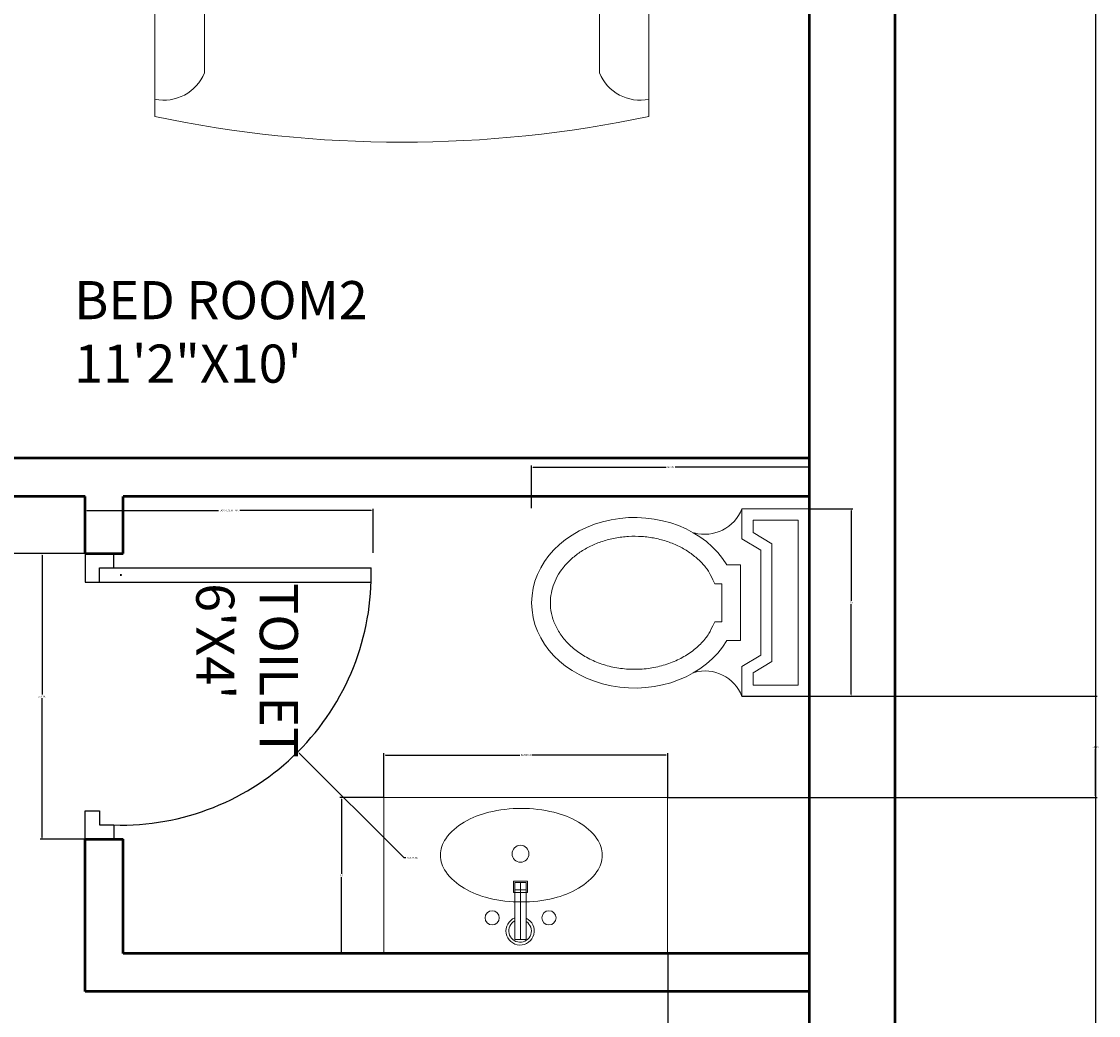
# Model space of a CAD drawing. Units: inches. Extents: x 1798 to 2141, y 1923 to 2386.
# Tile 8 of 9: x 2028 to 2141, y 2177 to 2281. Entities that reach past the tile are written whole.
import ezdxf

# ---------------------------------------------------------------- set-up
doc = ezdxf.new("R2010")
doc.units = ezdxf.units.IN
for name, color, linetype, lineweight in [('A-ANNO-DIMS', 2, 'Continuous', 18), ('A-AREA-IDEN', 7, 'Continuous', 25), ('A-FLOR-FIXT', 9, 'Continuous', 18), ('A-FURN', 8, 'Continuous', 13), ('door', 40, 'Continuous', 25), ('wall', 4, 'Continuous', 50)]:
    doc.layers.add(name, color=color, linetype=linetype, lineweight=lineweight)
doc.styles.get("Standard").update_dxf_attribs({"font": 'arial.ttf'})
doc.dimstyles.get("Standard").update_dxf_attribs({"dimtxt": 0.18, "dimasz": 0.18, "dimexe": 0.18, "dimexo": 0.0625, "dimgap": 0.09, "dimtad": 0, "dimtih": 1, "dimtoh": 1, "dimdec": 4, "dimzin": 0, "dimdsep": 46, "dimtxsty": 'Standard', "dimcen": 0.09, "dimadec": 0, "dimazin": 0, "dimtfac": 1, "dimtdec": 4, "dimtofl": 0, "dimtmove": 0, "dimatfit": 3, "dimfxl": 1, "dimtolj": 1, "dimtzin": 0, "dimarcsym": 0})

# ---------------------------------------------------------------- blocks, each defined once
blk = doc.blocks.new('A$C4F543DC7')
for p, q in [((0.2381, 3.1233, -0.4388), (0.2381, 3.3614, -0.4388)), ((3.0888, 3.1233, -0.4388), (3.0888, 3.3614, -0.4388)), ((0.0134, 3.35, -0.1688), (3.3134, 3.35, -0.1688)), ((0.4634, 3.35, -0.1688), (0.0134, 3.35, -0.1688)), ((0.0134, 2.896, -0.1688), (0.0134, 3.35, -0.1688)), ((0.0134, 3.35, -0.1688), (0.0134, 2.896, -0.1688)), ((0.4634, 3.35, -0.1688), (0.4634, 0.8, -0.1688)), ((2.8634, 3.35, -0.1688), (0.4634, 3.35, -0.1688)), ((0.4634, 2.896, -0.1688), (0.4634, 3.35, -0.1688)), ((2.8634, 0.8, -0.1688), (2.8634, 3.35, -0.1688)), ((2.8634, 3.35, -0.1688), (3.3134, 3.35, -0.1688)), ((2.8634, 2.896, -0.1688), (2.8634, 3.35, -0.1688)), ((3.3134, 3.35, -0.1688), (3.3134, 2.896, -0.1688)), ((3.3134, 3.35, -0.1688), (3.3134, 2.896, -0.1688)), ((1.5354, 3.226, -0.1688), (0.6684, 3.226, -0.1688)), ((2.6644, 3.226, -0.1688), (1.7974, 3.226, -0.1688)), ((0.2381, 3.1233, -0.4388), (0, 3.1233, -0.4388)), ((0.2381, 3.1233, -0.4388), (0.4762, 3.1233, -0.4388)), ((0.2381, 3.1233, -0.4388), (0.2381, 2.8852, -0.4388)), ((0.5684, 3.126, -0.1688), (0.5684, 2.884, -0.1688)), ((1.6354, 2.884, -0.1688), (1.6354, 3.126, -0.1688)), ((1.6974, 3.126, -0.1688), (1.6974, 2.884, -0.1688)), ((2.7644, 2.884, -0.1688), (2.7644, 3.126, -0.1688)), ((3.0888, 3.1233, -0.4388), (2.8507, 3.1233, -0.4388)), ((3.0888, 3.1233, -0.4388), (3.0888, 2.8852, -0.4388)), ((3.0888, 3.1233, -0.4388), (3.3269, 3.1233, -0.4388)), ((0.4634, 2.896, -0.1688), (0.0134, 2.896, -0.1688)), ((0.0134, 2.896, -0.1688), (0.4634, 2.896, -0.1688)), ((0.4634, 0.8, -0.1688), (0.4634, 2.896, -0.1688)), ((2.8634, 2.896, -0.1688), (2.8634, 0.8, -0.1688)), ((3.3134, 2.896, -0.1688), (2.8634, 2.896, -0.1688)), ((3.3134, 2.896, -0.1688), (2.8634, 2.896, -0.1688)), ((0.6684, 2.784, -0.1688), (1.5354, 2.784, -0.1688)), ((1.7974, 2.784, -0.1688), (2.6644, 2.784, -0.1688)), ((1.6534, 2.573, -0.1688), (0.5504, 2.025, -0.1688)), ((0.8414, 1.752, -0.1688), (1.6534, 2.573, -0.1688)), ((2.4814, 1.752, -0.1688), (1.6694, 2.573, -0.1688)), ((1.6694, 2.573, -0.1688), (2.7724, 2.025, -0.1688)), ((0.5504, 2.025, -0.1688), (0.8414, 1.752, -0.1688)), ((2.7724, 2.025, -0.1688), (2.4814, 1.752, -0.1688)), ((2.683, 1.312, -0.1688), (2.7182, 1.3641, -0.1688)), ((0.5369, 1.3267, -0.1688), (0.6088, 1.2835, -0.1688)), ((2.6479, 1.2774, -0.1688), (2.683, 1.312, -0.1688)), ((0.6088, 1.2835, -0.1688), (0.6756, 1.2566, -0.1688)), ((1.3963, 1.2612, -0.1688), (1.4328, 1.2664, -0.1688)), ((1.4328, 1.2664, -0.1688), (1.4679, 1.2677, -0.1688)), ((1.4679, 1.2677, -0.1688), (1.501, 1.2643, -0.1688)), ((1.8849, 1.263, -0.1688), (1.913, 1.2698, -0.1688)), ((1.913, 1.2698, -0.1688), (1.9397, 1.2722, -0.1688)), ((1.9397, 1.2722, -0.1688), (1.9649, 1.2692, -0.1688)), ((1.9649, 1.2692, -0.1688), (1.989, 1.2617, -0.1688)), ((2.6129, 1.257, -0.1688), (2.6479, 1.2774, -0.1688)), ((0.6756, 1.2566, -0.1688), (0.7373, 1.2428, -0.1688)), ((0.7373, 1.2428, -0.1688), (0.794, 1.239, -0.1688)), ((0.794, 1.239, -0.1688), (0.8457, 1.242, -0.1688)), ((0.8457, 1.242, -0.1688), (0.8925, 1.2489, -0.1688)), ((0.8925, 1.2489, -0.1688), (0.9345, 1.2564, -0.1688)), ((0.9345, 1.2564, -0.1688), (0.9718, 1.2615, -0.1688)), ((0.9718, 1.2615, -0.1688), (1.0044, 1.2617, -0.1688)), ((1.0044, 1.2617, -0.1688), (1.0334, 1.2578, -0.1688)), ((1.0334, 1.2578, -0.1688), (1.0597, 1.2509, -0.1688)), ((1.0597, 1.2509, -0.1688), (1.0842, 1.2424, -0.1688)), ((1.0842, 1.2424, -0.1688), (1.1081, 1.2336, -0.1688)), ((1.1081, 1.2336, -0.1688), (1.1322, 1.2257, -0.1688)), ((1.1322, 1.2257, -0.1688), (1.1577, 1.2201, -0.1688)), ((1.2163, 1.2204, -0.1688), (1.2498, 1.2264, -0.1688)), ((1.2498, 1.2264, -0.1688), (1.2852, 1.2347, -0.1688)), ((1.2852, 1.2347, -0.1688), (1.3218, 1.2441, -0.1688)), ((1.3218, 1.2441, -0.1688), (1.3591, 1.2533, -0.1688)), ((1.3591, 1.2533, -0.1688), (1.3963, 1.2612, -0.1688)), ((1.501, 1.2643, -0.1688), (1.5324, 1.257, -0.1688)), ((1.5324, 1.257, -0.1688), (1.5624, 1.2473, -0.1688)), ((1.5624, 1.2473, -0.1688), (1.5915, 1.2365, -0.1688)), ((1.5915, 1.2365, -0.1688), (1.6199, 1.2259, -0.1688)), ((1.6199, 1.2259, -0.1688), (1.6481, 1.2169, -0.1688)), ((1.7651, 1.2199, -0.1688), (1.7955, 1.2301, -0.1688)), ((1.7955, 1.2301, -0.1688), (1.8258, 1.2417, -0.1688)), ((1.8258, 1.2417, -0.1688), (1.8557, 1.2531, -0.1688)), ((1.8557, 1.2531, -0.1688), (1.8849, 1.263, -0.1688)), ((1.989, 1.2617, -0.1688), (2.0124, 1.2512, -0.1688)), ((2.0124, 1.2512, -0.1688), (2.0359, 1.2391, -0.1688)), ((2.0359, 1.2391, -0.1688), (2.0599, 1.2269, -0.1688)), ((2.0599, 1.2269, -0.1688), (2.0849, 1.216, -0.1688)), ((2.242, 1.2182, -0.1688), (2.2791, 1.2279, -0.1688)), ((2.2791, 1.2279, -0.1688), (2.3173, 1.2378, -0.1688)), ((2.3173, 1.2378, -0.1688), (2.3558, 1.2465, -0.1688)), ((2.3558, 1.2465, -0.1688), (2.3944, 1.2527, -0.1688)), ((2.3944, 1.2527, -0.1688), (2.4325, 1.255, -0.1688)), ((2.4325, 1.255, -0.1688), (2.4698, 1.2529, -0.1688)), ((2.4698, 1.2529, -0.1688), (2.5064, 1.2488, -0.1688)), ((2.5064, 1.2488, -0.1688), (2.5423, 1.2459, -0.1688)), ((2.5423, 1.2459, -0.1688), (2.5777, 1.2476, -0.1688)), ((2.5777, 1.2476, -0.1688), (2.6129, 1.257, -0.1688)), ((0.6743, 1.1706, -0.1688), (0.7364, 1.1825, -0.1688)), ((0.7364, 1.1825, -0.1688), (0.7931, 1.1846, -0.1688)), ((0.7931, 1.1846, -0.1688), (0.8447, 1.1799, -0.1688)), ((0.8447, 1.1799, -0.1688), (0.8913, 1.1716, -0.1688)), ((1.0831, 1.172, -0.1688), (1.1072, 1.18, -0.1688)), ((1.1072, 1.18, -0.1688), (1.1316, 1.1872, -0.1688)), ((1.1316, 1.1872, -0.1688), (1.1573, 1.192, -0.1688)), ((1.1573, 1.192, -0.1688), (1.1851, 1.1932, -0.1688)), ((1.1577, 1.2201, -0.1688), (1.1855, 1.218, -0.1688)), ((1.1851, 1.1932, -0.1688), (1.2158, 1.1898, -0.1688)), ((1.1855, 1.218, -0.1688), (1.2163, 1.2204, -0.1688)), ((1.2158, 1.1898, -0.1688), (1.2491, 1.1828, -0.1688)), ((1.2491, 1.1828, -0.1688), (1.2842, 1.1734, -0.1688)), ((1.6191, 1.1716, -0.1688), (1.6475, 1.1797, -0.1688)), ((1.6475, 1.1797, -0.1688), (1.676, 1.1849, -0.1688)), ((1.6481, 1.2169, -0.1688), (1.6765, 1.2108, -0.1688)), ((1.676, 1.1849, -0.1688), (1.7049, 1.1858, -0.1688)), ((1.6765, 1.2108, -0.1688), (1.7053, 1.209, -0.1688)), ((1.7049, 1.1858, -0.1688), (1.7344, 1.1816, -0.1688)), ((1.7053, 1.209, -0.1688), (1.7349, 1.2124, -0.1688)), ((1.7344, 1.1816, -0.1688), (1.7643, 1.1731, -0.1688)), ((1.7349, 1.2124, -0.1688), (1.7651, 1.2199, -0.1688)), ((2.0849, 1.216, -0.1688), (2.1117, 1.2077, -0.1688)), ((2.1112, 1.1743, -0.1688), (2.1403, 1.1775, -0.1688)), ((2.1117, 1.2077, -0.1688), (2.1407, 1.2037, -0.1688)), ((2.1403, 1.1775, -0.1688), (2.1718, 1.1755, -0.1688)), ((2.1407, 1.2037, -0.1688), (2.1723, 1.2047, -0.1688)), ((2.1723, 1.2047, -0.1688), (2.2062, 1.21, -0.1688)), ((2.2062, 1.21, -0.1688), (2.242, 1.2182, -0.1688)), ((0.5334, 1.105, -0.1688), (0.6067, 1.1458, -0.1688)), ((0.6067, 1.1458, -0.1688), (0.6743, 1.1706, -0.1688)), ((0.8913, 1.1716, -0.1688), (0.9331, 1.1628, -0.1688)), ((0.9331, 1.1628, -0.1688), (0.9701, 1.1565, -0.1688)), ((0.9701, 1.1565, -0.1688), (1.0027, 1.1552, -0.1688)), ((1.0027, 1.1552, -0.1688), (1.0318, 1.1582, -0.1688)), ((1.0318, 1.1582, -0.1688), (1.0583, 1.1642, -0.1688)), ((1.0583, 1.1642, -0.1688), (1.0831, 1.172, -0.1688)), ((1.2842, 1.1734, -0.1688), (1.3206, 1.1629, -0.1688)), ((1.3206, 1.1629, -0.1688), (1.3575, 1.1524, -0.1688)), ((1.3575, 1.1524, -0.1688), (1.3945, 1.1434, -0.1688)), ((1.3945, 1.1434, -0.1688), (1.4308, 1.1371, -0.1688)), ((1.4308, 1.1371, -0.1688), (1.4658, 1.1347, -0.1688)), ((1.4658, 1.1347, -0.1688), (1.499, 1.137, -0.1688)), ((1.499, 1.137, -0.1688), (1.5306, 1.1433, -0.1688)), ((1.5306, 1.1433, -0.1688), (1.5609, 1.152, -0.1688)), ((1.5609, 1.152, -0.1688), (1.5903, 1.1619, -0.1688)), ((1.5903, 1.1619, -0.1688), (1.6191, 1.1716, -0.1688)), ((1.7643, 1.1731, -0.1688), (1.7944, 1.1619, -0.1688)), ((1.7944, 1.1619, -0.1688), (1.8244, 1.1494, -0.1688)), ((1.8244, 1.1494, -0.1688), (1.8539, 1.137, -0.1688)), ((1.8539, 1.137, -0.1688), (1.8827, 1.1263, -0.1688)), ((1.9868, 1.1243, -0.1688), (2.0106, 1.134, -0.1688)), ((2.0106, 1.134, -0.1688), (2.0344, 1.1454, -0.1688)), ((2.0344, 1.1454, -0.1688), (2.0588, 1.1568, -0.1688)), ((2.0588, 1.1568, -0.1688), (2.0842, 1.167, -0.1688)), ((2.0842, 1.167, -0.1688), (2.1112, 1.1743, -0.1688)), ((2.1718, 1.1755, -0.1688), (2.2056, 1.1691, -0.1688)), ((2.2056, 1.1691, -0.1688), (2.2411, 1.1598, -0.1688)), ((2.2411, 1.1598, -0.1688), (2.2779, 1.1489, -0.1688)), ((2.2779, 1.1489, -0.1688), (2.3157, 1.1379, -0.1688)), ((2.3157, 1.1379, -0.1688), (2.354, 1.1279, -0.1688)), ((1.8827, 1.1263, -0.1688), (1.9106, 1.1186, -0.1688)), ((1.9106, 1.1186, -0.1688), (1.9373, 1.1153, -0.1688)), ((1.9373, 1.1153, -0.1688), (1.9625, 1.1176, -0.1688)), ((1.9625, 1.1176, -0.1688), (1.9868, 1.1243, -0.1688)), ((2.354, 1.1279, -0.1688), (2.3923, 1.1205, -0.1688)), ((2.3923, 1.1205, -0.1688), (2.4304, 1.117, -0.1688)), ((2.4304, 1.117, -0.1688), (2.4677, 1.118, -0.1688)), ((2.4677, 1.118, -0.1688), (2.5043, 1.1209, -0.1688)), ((2.5043, 1.1209, -0.1688), (2.5403, 1.1226, -0.1688)), ((2.5403, 1.1226, -0.1688), (2.5757, 1.1199, -0.1688)), ((2.5757, 1.1199, -0.1688), (2.6106, 1.1094, -0.1688)), ((2.6106, 1.1094, -0.1688), (2.645, 1.0879, -0.1688)), ((2.645, 1.0879, -0.1688), (2.6789, 1.0522, -0.1688)), ((2.6789, 1.0522, -0.1688), (2.7124, 0.999, -0.1688)), ((0.4634, 0.85, -0.1688), (2.8634, 0.85, -0.1688)), ((0.4634, 0.8, -0.1688), (2.8634, 0.8, -0.1688)), ((0.6634, 0.8, -0.1688), (0.4634, 0.8, -0.1688)), ((0.6634, 0.8, -0.1688), (2.6634, 0.8, -0.1688)), ((0.6634, 0.104, -0.1688), (0.6634, 0.8, -0.1688)), ((0.6634, 0.104, -0.1688), (0.6634, 0.8, -0.1688)), ((0.8634, 0.281, -0.1688), (0.8634, 0.8, -0.1688)), ((2.4634, 0.8, -0.1688), (2.4634, 0.281, -0.1688)), ((2.8634, 0.8, -0.1688), (2.6634, 0.8, -0.1688)), ((2.6634, 0.8, -0.1688), (2.6634, 0.104, -0.1688)), ((2.6634, 0.8, -0.1688), (2.6634, 0.104, -0.1688))]:
    blk.add_line(p, q)
for centre, radius in [((0.2381, 3.1233, -0.4388), 0.139), ((3.0888, 3.1233, -0.4388), 0.139), ((0.2381, 3.1233, -0.4388), 0.075), ((3.0888, 3.1233, -0.4388), 0.075)]:
    blk.add_circle(centre, radius)
for centre, radius, start, end in [((0.6684, 3.126, -0.1688), 0.1, 90, 180), ((1.5354, 3.126, -0.1688), 0.1, 0, 90), ((1.7974, 3.126, -0.1688), 0.1, 90, 180), ((2.6644, 3.126, -0.1688), 0.1, 0, 90), ((0.6684, 2.884, -0.1688), 0.1, 180, 270), ((1.5354, 2.884, -0.1688), 0.1, 270, 0), ((1.7974, 2.884, -0.1688), 0.1, 180, 270), ((2.6644, 2.884, -0.1688), 0.1, 270, 0), ((0.6994, 0.3472, -0.1688), 0.1769, 258.2616, 338.032), ((2.6275, 0.3472, -0.1688), 0.1769, 201.968, 281.7384), ((1.6634, 4.8597, -0.1688), 4.8597, 258.1252, 281.8748), ((1.6634, 4.8597, -0.1688), 4.8597, 258.1252, 281.8748)]:
    blk.add_arc(centre, radius, start, end)
blk = doc.blocks.new('A$C7C8779AE')
for p, q in [((0, 0.7405), (0, 0.5605)), ((0.5, 0.7405), (0, 0.7405)), ((0.5, 0.5605), (0.5, 0.7405)), ((0.47, 0.7105), (0.03, 0.7105)), ((0.03, 0.7105), (0.03, 0.5905)), ((0.47, 0.5905), (0.47, 0.7105)), ((0.093, 0.6405), (0.063, 0.5905)), ((0.093, 0.6405), (0.407, 0.6405)), ((0.437, 0.5905), (0.407, 0.6405)), ((0.11, 0.6105), (0.08, 0.5605)), ((0.11, 0.6105), (0.39, 0.6105)), ((0.42, 0.5605), (0.39, 0.6105)), ((0.03, 0.5905), (0.063, 0.5905)), ((0.437, 0.5905), (0.47, 0.5905)), ((0, 0.5605), (0.08, 0.5605)), ((0.1497, 0.557), (0.1497, 0.5203)), ((0.1497, 0.557), (0.3514, 0.557)), ((0.3514, 0.557), (0.3514, 0.5203)), ((0.42, 0.5605), (0.5, 0.5605)), ((0.1997, 0.507), (0.1997, 0.4879)), ((0.1997, 0.507), (0.3014, 0.507)), ((0.3014, 0.507), (0.3014, 0.4879))]:
    blk.add_line(p, q)
for centre, start, end in [((-0.0386, 0.4613), 344.642, 68.7339), ((0.5386, 0.4613), 111.2661, 195.358)]:
    blk.add_arc(centre, 0.1064, start, end)
blk.add_ellipse((0.2506, 0.2744), major_axis=(0, 0.2744), ratio=0.828948, start_param=0.459479, end_param=5.823706)
blk.add_open_spline([(0.1997, 0.4879), (0.1697, 0.474), (0.1642, 0.4702), (0.1512, 0.4602), (0.1438, 0.4535), (0.1298, 0.4388), (0.1233, 0.4306), (0.1111, 0.4131), (0.1055, 0.4037), (0.0956, 0.3838), (0.0912, 0.3733), (0.0838, 0.3516), (0.0808, 0.3403), (0.0762, 0.3172), (0.0746, 0.3055), (0.073, 0.2817), (0.0729, 0.2698), (0.0743, 0.246), (0.0758, 0.2342), (0.0801, 0.2111), (0.0831, 0.1998), (0.0903, 0.1779), (0.0945, 0.1673), (0.1043, 0.1473), (0.1098, 0.1378), (0.1218, 0.12), (0.1283, 0.1118), (0.1421, 0.0968), (0.1494, 0.09), (0.1646, 0.078), (0.1725, 0.0728), (0.1887, 0.064), (0.1969, 0.0603), (0.2137, 0.0547), (0.2222, 0.0527), (0.2392, 0.0502), (0.2478, 0.0498), (0.2664, 0.0505), (0.2764, 0.052), (0.2963, 0.0573), (0.3061, 0.061), (0.3253, 0.0707), (0.3346, 0.0766), (0.3525, 0.0906), (0.3611, 0.0987), (0.3771, 0.1169), (0.3845, 0.127), (0.3978, 0.1488), (0.4037, 0.1605), (0.4137, 0.1853), (0.4178, 0.1983), (0.424, 0.2251), (0.4261, 0.2389), (0.4282, 0.2668), (0.4283, 0.2809), (0.4262, 0.3088), (0.4241, 0.3226), (0.418, 0.3495), (0.414, 0.3625), (0.404, 0.3873), (0.3982, 0.3991), (0.385, 0.421), (0.3776, 0.4311), (0.3617, 0.4494), (0.3531, 0.4575), (0.3382, 0.4693), (0.3321, 0.4736), (0.3014, 0.4879)], degree=3, knots=[0.459479, 0.459479, 0.459479, 0.459479, 0.567422, 0.567422, 0.720865, 0.720865, 0.874307, 0.874307, 1.02775, 1.02775, 1.181192, 1.181192, 1.334635, 1.334635, 1.488077, 1.488077, 1.64152, 1.64152, 1.794963, 1.794963, 1.948405, 1.948405, 2.101848, 2.101848, 2.25529, 2.25529, 2.408733, 2.408733, 2.562175, 2.562175, 2.715618, 2.715618, 2.86906, 2.86906, 3.022503, 3.022503, 3.175946, 3.175946, 3.356457, 3.356457, 3.536968, 3.536968, 3.717479, 3.717479, 3.89799, 3.89799, 4.078501, 4.078501, 4.259012, 4.259012, 4.439523, 4.439523, 4.620035, 4.620035, 4.800546, 4.800546, 4.981057, 4.981057, 5.161568, 5.161568, 5.342079, 5.342079, 5.52259, 5.52259, 5.703101, 5.703101, 5.823706, 5.823706, 5.823706, 5.823706])
blk = doc.blocks.new('A$C50A015BB')
for p, q in [((0, 0.55), (1, 0.55)), ((0, 0.55), (0, 0)), ((1, 0.55), (1, 0)), ((0.4985, 0.5), (0.5385, 0.5)), ((0.4985, 0.5), (0.4985, 0.3)), ((0.5185, 0.5), (0.5185, 0.3)), ((0.5385, 0.5), (0.5385, 0.3)), ((0.4935, 0.335), (0.4935, 0.295)), ((0.4935, 0.335), (0.5435, 0.335)), ((0.4985, 0.325), (0.5385, 0.325)), ((0.5435, 0.335), (0.5435, 0.295)), ((0.4935, 0.295), (0.5435, 0.295)), ((0.4985, 0.3), (0.5385, 0.3)), ((0, 0), (1, 0)), ((0, 0), (1, 0))]:
    blk.add_line(p, q)
for centre, radius in [((0.4185, 0.424), 0.025), ((0.6185, 0.424), 0.025), ((0.5185, 0.1981), 0.0298)]:
    blk.add_circle(centre, radius)
for centre, radius, start, end in [((0.5201, 0.4703), 0.0497, 291.7425, 244.2331), ((0.5201, 0.4703), 0.0397, 297.632, 237.0256), ((0.4772, 0.0383), 0.3252, 103.4853, 120.0686), ((0.5157, -0.1225), 0.4906, 90, 103.4853), ((0.5157, -0.1225), 0.4906, 76.5147, 90), ((0.5543, 0.0383), 0.3252, 59.9314, 76.5147), ((0.4185, 0.1397), 0.2081, 120.0686, 144.4178), ((0.613, 0.1397), 0.2081, 35.5822, 59.9314), ((0.3299, 0.2031), 0.0991, 144.4178, 180), ((0.7016, 0.2031), 0.0991, 0, 35.5822), ((0.3299, 0.2031), 0.0991, 180, 215.5822), ((0.7016, 0.2031), 0.0991, 324.4178, 0), ((0.4185, 0.2665), 0.2081, 215.5822, 239.9314), ((0.613, 0.2665), 0.2081, 300.0686, 324.4178), ((0.4772, 0.3679), 0.3252, 239.9314, 256.5147), ((0.5543, 0.3679), 0.3252, 283.4853, 300.0686), ((0.5157, 0.5288), 0.4906, 256.5147, 270), ((0.5157, 0.5288), 0.4906, 270, 283.4853)]:
    blk.add_arc(centre, radius, start, end)
blk = doc.blocks.new('DOOR-SWING-30IN')
for p, q in [((3, 30), (0, 30)), ((0, 30), (0, 27)), ((3, 28.5), (3, 30)), ((1.5, 27), (1.5, 28.5)), ((1.5, 28.5), (3, 28.5)), ((1.5, 28.5), (30, 28.5)), ((0, 27), (1.5, 27)), ((0, 27), (30, 27)), ((0, 0), (0, 3)), ((0, 3), (1.5, 3)), ((1.5, 3), (1.5, 1.5)), ((1.5, 1.5), (3, 1.5)), ((3, 1.5), (3, 0)), ((3, 0), (0, 0))]:
    blk.add_line(p, q)
blk.add_arc((3.75, 27.75), 26.26, 268.3634, 1.6366)
blk = doc.blocks.new('*D21')
at = {"layer": 'A-ANNO-DIMS', "color": 0, "lineweight": -2, "transparency": 16777216}
for p, q in [((2034.51, 2225.39), (2034.51, 2230.03)), ((2034.69, 2229.85), (2048.49, 2229.85)), ((2064.54, 2229.85), (2050.75, 2229.85)), ((2064.72, 2225.39), (2064.72, 2230.03))]:
    blk.add_line(p, q, dxfattribs=at)
at = {"layer": 'A-ANNO-DIMS', "color": 0, "transparency": 16777216}
for points in [[(2034.69, 2229.88), (2034.69, 2229.82), (2034.51, 2229.85)], [(2064.54, 2229.88), (2064.54, 2229.82), (2064.72, 2229.85)]]:
    blk.add_solid(points, dxfattribs=at)
at = {"layer": 'Defpoints', "color": 0, "transparency": 16777216}
for p in [(2064.72, 2229.85), (2034.51, 2225.32), (2064.72, 2225.32)]:
    blk.add_point(p, dxfattribs=at)
at = {"layer": 'A-ANNO-DIMS', "color": 0, "transparency": 16777216, "insert": (2049.62, 2229.85), "char_height": 0.18, "attachment_point": 5}
blk.add_mtext('\\A1;DOOR D2 30 TYP.', dxfattribs=at)
blk = doc.blocks.new('*D22')
at = {"layer": 'A-ANNO-DIMS', "color": 0, "lineweight": -2, "transparency": 16777216}
for p, q in [((2034.45, 2225.32), (2029.8, 2225.32)), ((2029.98, 2225.14), (2029.98, 2210.51)), ((2029.98, 2195.5), (2029.98, 2210.14)), ((2034.45, 2195.32), (2029.8, 2195.32))]:
    blk.add_line(p, q, dxfattribs=at)
at = {"layer": 'A-ANNO-DIMS', "color": 0, "transparency": 16777216}
for points in [[(2029.95, 2225.14), (2030.01, 2225.14), (2029.98, 2225.32)], [(2029.95, 2195.5), (2030.01, 2195.5), (2029.98, 2195.32)]]:
    blk.add_solid(points, dxfattribs=at)
at = {"layer": 'Defpoints', "color": 0, "transparency": 16777216}
for p in [(2029.98, 2225.32), (2034.51, 2225.32), (2034.51, 2195.32)]:
    blk.add_point(p, dxfattribs=at)
at = {"layer": 'A-ANNO-DIMS', "color": 0, "transparency": 16777216, "insert": (2029.98, 2210.32), "char_height": 0.18, "attachment_point": 5}
blk.add_mtext('\\A1;30 TYP.', dxfattribs=at)
blk = doc.blocks.new('*D25')
at = {"layer": 'A-ANNO-DIMS', "color": 0, "lineweight": -2, "transparency": 16777216}
for p, q in [((2081.36, 2230.08), (2081.36, 2234.57)), ((2081.54, 2234.39), (2095.47, 2234.39)), ((2110.33, 2234.39), (2096.41, 2234.39)), ((2110.51, 2230.08), (2110.51, 2234.57))]:
    blk.add_line(p, q, dxfattribs=at)
at = {"layer": 'A-ANNO-DIMS', "color": 0, "transparency": 16777216}
for points in [[(2081.54, 2234.42), (2081.54, 2234.36), (2081.36, 2234.39)], [(2110.33, 2234.42), (2110.33, 2234.36), (2110.51, 2234.39)]]:
    blk.add_solid(points, dxfattribs=at)
at = {"layer": 'Defpoints', "color": 0, "transparency": 16777216}
for p in [(2110.51, 2234.39), (2081.36, 2230.01), (2110.51, 2230.01)]:
    blk.add_point(p, dxfattribs=at)
at = {"layer": 'A-ANNO-DIMS', "color": 0, "transparency": 16777216, "insert": (2095.94, 2234.39), "char_height": 0.18, "attachment_point": 5}
blk.add_mtext('\\A1;WC 29', dxfattribs=at)
blk = doc.blocks.new('*D26')
at = {"layer": 'A-ANNO-DIMS', "color": 0, "lineweight": -2, "transparency": 16777216}
for p, q in [((2110.58, 2230.01), (2115.07, 2230.01)), ((2114.89, 2229.83), (2114.89, 2220.35)), ((2114.89, 2210.51), (2114.89, 2219.99)), ((2110.58, 2210.33), (2115.07, 2210.33))]:
    blk.add_line(p, q, dxfattribs=at)
at = {"layer": 'A-ANNO-DIMS', "color": 0, "transparency": 16777216}
for points in [[(2114.86, 2229.83), (2114.92, 2229.83), (2114.89, 2230.01)], [(2114.86, 2210.51), (2114.92, 2210.51), (2114.89, 2210.33)]]:
    blk.add_solid(points, dxfattribs=at)
at = {"layer": 'Defpoints', "color": 0, "transparency": 16777216}
for p in [(2110.51, 2230.01), (2110.51, 2210.33), (2114.89, 2210.33)]:
    blk.add_point(p, dxfattribs=at)
at = {"layer": 'A-ANNO-DIMS', "color": 0, "transparency": 16777216, "insert": (2114.89, 2220.17), "char_height": 0.18, "attachment_point": 5}
blk.add_mtext('\\A1;20', dxfattribs=at)
blk = doc.blocks.new('*D27')
at = {"layer": 'A-ANNO-DIMS', "color": 0, "lineweight": -2, "transparency": 16777216}
for p, q in [((2065.86, 2199.76), (2065.86, 2204.35)), ((2066.04, 2204.17), (2080.12, 2204.17)), ((2095.46, 2204.17), (2081.38, 2204.17)), ((2095.64, 2199.76), (2095.64, 2204.35))]:
    blk.add_line(p, q, dxfattribs=at)
at = {"layer": 'A-ANNO-DIMS', "color": 0, "transparency": 16777216}
for points in [[(2066.04, 2204.2), (2066.04, 2204.14), (2065.86, 2204.17)], [(2095.46, 2204.2), (2095.46, 2204.14), (2095.64, 2204.17)]]:
    blk.add_solid(points, dxfattribs=at)
at = {"layer": 'Defpoints', "color": 0, "transparency": 16777216}
for p in [(2065.86, 2204.17), (2065.86, 2199.7), (2095.64, 2199.7)]:
    blk.add_point(p, dxfattribs=at)
at = {"layer": 'A-ANNO-DIMS', "color": 0, "transparency": 16777216, "insert": (2080.75, 2204.17), "char_height": 0.18, "attachment_point": 5}
blk.add_mtext('\\A1;BASIN 30', dxfattribs=at)
blk = doc.blocks.new('*D28')
at = {"layer": 'A-ANNO-DIMS', "color": 0, "lineweight": -2, "transparency": 16777216}
for p, q in [((2065.8, 2199.7), (2061.22, 2199.7)), ((2061.4, 2199.52), (2061.4, 2191.69)), ((2061.4, 2183.5), (2061.4, 2191.33)), ((2065.8, 2183.32), (2061.22, 2183.32))]:
    blk.add_line(p, q, dxfattribs=at)
at = {"layer": 'A-ANNO-DIMS', "color": 0, "transparency": 16777216}
for points in [[(2061.37, 2199.52), (2061.43, 2199.52), (2061.4, 2199.7)], [(2061.37, 2183.5), (2061.43, 2183.5), (2061.4, 2183.32)]]:
    blk.add_solid(points, dxfattribs=at)
at = {"layer": 'Defpoints', "color": 0, "transparency": 16777216}
for p in [(2065.86, 2199.7), (2061.4, 2183.32), (2065.86, 2183.32)]:
    blk.add_point(p, dxfattribs=at)
at = {"layer": 'A-ANNO-DIMS', "color": 0, "transparency": 16777216, "insert": (2061.4, 2191.51), "char_height": 0.18, "attachment_point": 5}
blk.add_mtext('\\A1;16', dxfattribs=at)
blk = doc.blocks.new('*D32')
at = {"layer": 'A-ANNO-DIMS', "color": 0, "lineweight": -2, "transparency": 16777216}
for p, q in [((2119.58, 2364.32), (2140.72, 2364.32)), ((2140.54, 2364.14), (2140.54, 2154.51)), ((2140.54, 1944.5), (2140.54, 2154.14)), ((2119.58, 1944.32), (2140.72, 1944.32))]:
    blk.add_line(p, q, dxfattribs=at)
at = {"layer": 'A-ANNO-DIMS', "color": 0, "transparency": 16777216}
for points in [[(2140.51, 2364.14), (2140.57, 2364.14), (2140.54, 2364.32)], [(2140.51, 1944.5), (2140.57, 1944.5), (2140.54, 1944.32)]]:
    blk.add_solid(points, dxfattribs=at)
at = {"layer": 'Defpoints', "color": 0, "transparency": 16777216}
for p in [(2119.51, 2364.32), (2140.54, 2364.32), (2119.51, 1944.32)]:
    blk.add_point(p, dxfattribs=at)
at = {"layer": 'A-ANNO-DIMS', "color": 0, "transparency": 16777216, "insert": (2140.54, 2154.32), "char_height": 0.18, "attachment_point": 5}
blk.add_mtext('\\A1;420', dxfattribs=at)
blk = doc.blocks.new('*D37')
at = {"layer": 'A-ANNO-DIMS', "color": 0, "lineweight": -2, "transparency": 16777216}
for p, q in [((2034.45, 2231.32), (1798.31, 2231.32)), ((1798.49, 2231.14), (1798.49, 2228.51)), ((1798.49, 2225.5), (1798.49, 2228.14)), ((2034.45, 2225.32), (1798.31, 2225.32))]:
    blk.add_line(p, q, dxfattribs=at)
at = {"layer": 'A-ANNO-DIMS', "color": 0, "transparency": 16777216}
for points in [[(1798.46, 2231.14), (1798.52, 2231.14), (1798.49, 2231.32)], [(1798.46, 2225.5), (1798.52, 2225.5), (1798.49, 2225.32)]]:
    blk.add_solid(points, dxfattribs=at)
at = {"layer": 'Defpoints', "color": 0, "transparency": 16777216}
for p in [(1798.49, 2231.32), (2034.51, 2231.32), (2034.51, 2225.32)]:
    blk.add_point(p, dxfattribs=at)
at = {"layer": 'A-ANNO-DIMS', "color": 0, "transparency": 16777216, "insert": (1798.49, 2228.32), "char_height": 0.18, "attachment_point": 5}
blk.add_mtext('\\A1;6', dxfattribs=at)
blk = doc.blocks.new('*D48')
at = {"layer": 'A-ANNO-DIMS', "color": 0, "lineweight": -2, "transparency": 16777216}
for p, q in [((2095.64, 2183.26), (2095.64, 1923.12)), ((2110.51, 2183.26), (2110.51, 1923.12)), ((2095.82, 1923.3), (2102.62, 1923.3)), ((2110.33, 1923.3), (2103.53, 1923.3))]:
    blk.add_line(p, q, dxfattribs=at)
at = {"layer": 'A-ANNO-DIMS', "color": 0, "transparency": 16777216}
for points in [[(2095.82, 1923.33), (2095.82, 1923.27), (2095.64, 1923.3)], [(2110.33, 1923.33), (2110.33, 1923.27), (2110.51, 1923.3)]]:
    blk.add_solid(points, dxfattribs=at)
at = {"layer": 'Defpoints', "color": 0, "transparency": 16777216}
for p in [(2095.64, 2183.32), (2110.51, 2183.32), (2110.51, 1923.3)]:
    blk.add_point(p, dxfattribs=at)
at = {"layer": 'A-ANNO-DIMS', "color": 0, "transparency": 16777216, "insert": (2103.08, 1923.3), "char_height": 0.18, "attachment_point": 5}
blk.add_mtext('\\A1;14.878', dxfattribs=at)
blk = doc.blocks.new('*D49')
at = {"layer": 'A-ANNO-DIMS', "color": 0, "lineweight": -2, "transparency": 16777216}
for p, q in [((2103.49, 2210.33), (2140.72, 2210.33)), ((2140.54, 2210.15), (2140.54, 2205.2)), ((2140.54, 2199.88), (2140.54, 2204.83)), ((2095.7, 2199.7), (2140.72, 2199.7))]:
    blk.add_line(p, q, dxfattribs=at)
at = {"layer": 'A-ANNO-DIMS', "color": 0, "transparency": 16777216}
for points in [[(2140.51, 2210.15), (2140.57, 2210.15), (2140.54, 2210.33)], [(2140.51, 2199.88), (2140.57, 2199.88), (2140.54, 2199.7)]]:
    blk.add_solid(points, dxfattribs=at)
at = {"layer": 'Defpoints', "color": 0, "transparency": 16777216}
for p in [(2103.43, 2210.33), (2140.54, 2210.33), (2095.64, 2199.7)]:
    blk.add_point(p, dxfattribs=at)
at = {"layer": 'A-ANNO-DIMS', "color": 0, "transparency": 16777216, "insert": (2140.54, 2205.01), "char_height": 0.18, "attachment_point": 5}
blk.add_mtext('\\A1;10.63', dxfattribs=at)
blk = doc.blocks.new('*D52')
at = {"layer": 'A-ANNO-DIMS', "color": 0, "lineweight": -2, "transparency": 16777216}
for p, q in [((2038.17, 2223.07), (2038.35, 2223.07)), ((2038.26, 2222.98), (2038.26, 2223.16)), ((2067.97, 2193.36), (2056.96, 2204.38)), ((2068.15, 2193.36), (2067.97, 2193.36))]:
    blk.add_line(p, q, dxfattribs=at)
at = {"layer": 'A-ANNO-DIMS', "color": 0, "transparency": 16777216}
blk.add_solid([(2056.98, 2204.4), (2056.94, 2204.36), (2056.83, 2204.5)], dxfattribs=at)
at = {"layer": 'Defpoints', "color": 0, "transparency": 16777216}
for p in [(2038.26, 2223.07), (2056.83, 2204.5)]:
    blk.add_point(p, dxfattribs=at)
at = {"layer": 'A-ANNO-DIMS', "color": 0, "transparency": 16777216, "insert": (2068.83, 2193.36), "char_height": 0.18, "attachment_point": 5}
blk.add_mtext('\\A1;2X R26.26', dxfattribs=at)

msp = doc.modelspace()

# ---------------------------------------------------------------- linework, layer by layer
at = {"layer": 'wall'}
for p, q in [((2119.5141, 1944.3239), (2119.5141, 2364.3239)), ((2110.5141, 1944.3239), (2110.5141, 2355.3239)), ((2110.5141, 2235.3239), (2018.5141, 2235.3239)), ((2034.5141, 2231.3239), (2018.5141, 2231.3239)), ((2034.5141, 2225.3239), (2034.5141, 2231.3239)), ((2034.5141, 2225.3239), (2034.5141, 2231.3239)), ((2110.5141, 2231.3239), (2038.5141, 2231.3239)), ((2038.5141, 2225.3239), (2038.5141, 2231.3239)), ((2038.5141, 2225.3239), (2038.5141, 2231.3239)), ((2034.5141, 2225.3239), (2038.5141, 2225.3239)), ((2034.5141, 2179.3239), (2034.5141, 2195.3239)), ((2034.5141, 2195.3239), (2038.5141, 2195.3239)), ((2038.5141, 2183.3239), (2038.5141, 2195.3239)), ((2038.5141, 2183.3239), (2038.5141, 2195.3239)), ((2110.5141, 2183.3239), (2038.5141, 2183.3239)), ((2038.5141, 2179.3239), (2034.5141, 2179.3239)), ((2110.5141, 2179.3239), (2038.5141, 2179.3239))]:
    msp.add_line(p, q, dxfattribs=at)

# ---------------------------------------------------------------- block references
at = {"layer": 'A-FLOR-FIXT'}
for name, p, xscale, yscale, zscale, rotation in [('A$C7C8779AE', (2081.362, 2230.0147), 39.37007874015748, 39.37007874015748, 39.37007874015748, 270.0000000000037), ('A$C50A015BB', (2095.6365, 2199.7003), 29.77521223549502, 29.77521223549502, 29.77521223549502, 180)]:
    msp.add_blockref(name, p, dxfattribs=dict(at, xscale=xscale, yscale=yscale, zscale=zscale, rotation=rotation))
at = {"layer": 'A-FURN', "xscale": 25.91562772622874, "yscale": 25.91562772622874, "zscale": 25.91562772622874}
msp.add_blockref('A$C4F543DC7', (2024.6443, 2268.5065, 4.3733), dxfattribs=at)
at = {"layer": 'door'}
msp.add_blockref('DOOR-SWING-30IN', (2034.5141, 2195.3239), dxfattribs=at)

# ---------------------------------------------------------------- texts
at = {"layer": 'A-AREA-IDEN', "insert": (2033.3633, 2253.9265), "char_height": 4, "attachment_point": 1}
msp.add_mtext_dynamic_manual_height_columns('\\pxt7;BED ROOM2\\P11\'2"X10\'', width=35.513916, gutter_width=12.5, heights=[0], dxfattribs=at)
at = {"layer": 'A-AREA-IDEN', "insert": (2056.8332, 2222.2091), "char_height": 4, "attachment_point": 1, "rotation": 270}
msp.add_mtext_dynamic_manual_height_columns("TOILET\\P6'X4'", width=35.513916, gutter_width=12.5, heights=[0], dxfattribs=at)

# ---------------------------------------------------------------- dimensions: what is measured, and where the dimension line sits
at = {"layer": 'A-ANNO-DIMS'}
for base, p1, p2, angle, override, picture, middle in [((2140.5391, 2364.3239), (2119.5141, 1944.3239), (2119.5141, 2364.3239), 90, {"dimdec": 0, "dimlfac": 1, "dimrnd": 0, "dimzin": 0, "dimdsep": 46, "dimlunit": 2}, '*D32', (2140.5391, 2154.3239)), ((1798.4891, 2231.3239), (2034.5141, 2225.3239), (2034.5141, 2231.3239), 90, {"dimdec": 0, "dimlfac": 1, "dimrnd": 0, "dimzin": 0, "dimdsep": 46, "dimlunit": 2}, '*D37', (1798.4891, 2228.3239)), ((2114.8869, 2210.3296), (2110.5141, 2230.0147), (2110.5141, 2210.3296), 270, {"dimdec": 0, "dimlfac": 1, "dimrnd": 0, "dimzin": 0, "dimdsep": 46, "dimlunit": 2}, '*D26', (2114.8869, 2220.1722)), ((2140.5391, 2210.3296), (2095.6365, 2199.7003), (2103.4275, 2210.3296), 90, {"dimdec": 2, "dimlfac": 1, "dimrnd": 0, "dimzin": 0, "dimdsep": 46, "dimlunit": 2}, '*D49', (2140.5391, 2205.015)), ((2061.395, 2183.3239), (2065.8613, 2199.7003), (2065.8613, 2183.3239), 270, {"dimdec": 0, "dimlfac": 1, "dimrnd": 0, "dimzin": 0, "dimdsep": 46, "dimlunit": 2}, '*D28', (2061.395, 2191.5121))]:
    dim = msp.add_linear_dim(base=base, p1=p1, p2=p2, angle=angle, dimstyle='Standard', override=override, dxfattribs=at)
    dim.commit()
    dim.dimension.update_dxf_attribs({"geometry": picture, "text_midpoint": middle})
for base, p1, p2, angle, text, picture, middle in [((2110.5141, 2234.3875), (2081.362, 2230.0147), (2110.5141, 2230.0147), 0, 'WC <>', '*D25', (2095.9381, 2234.3875)), ((2029.9832, 2225.3239), (2034.5141, 2195.3239), (2034.5141, 2225.3239), 90, '<> TYP.', '*D22', (2029.9832, 2210.3239)), ((2065.8613, 2204.1665), (2095.6365, 2199.7003), (2065.8613, 2199.7003), 180, 'BASIN <>', '*D27', (2080.7489, 2204.1665))]:
    dim = msp.add_linear_dim(base=base, p1=p1, p2=p2, angle=angle, text=text, dimstyle='Standard', override={"dimdec": 0, "dimlfac": 1, "dimrnd": 0, "dimzin": 0, "dimdsep": 46, "dimlunit": 2}, dxfattribs=at)
    dim.commit()
    dim.dimension.update_dxf_attribs({"geometry": picture, "text_midpoint": middle})
dim = msp.add_linear_dim(base=(2064.7205, 2229.8548), p1=(2034.5141, 2225.3239), p2=(2064.7205, 2225.3239), text='DOOR D2 <> TYP.', dimstyle='Standard', override={"dimdec": 0, "dimlfac": 1, "dimrnd": 0, "dimzin": 0, "dimdsep": 46, "dimlunit": 2}, dxfattribs=at)
dim.commit()
dim.dimension.update_dxf_attribs({"geometry": '*D21', "text_midpoint": (2049.6173, 2229.8548)})
dim = msp.add_radius_dim(center=(2038.2641, 2223.0739), mpoint=(2056.8332, 2204.5048), text='2X <>', dimstyle='Standard', override={"dimdec": 2, "dimlfac": 1, "dimrnd": 0, "dimzin": 0, "dimdsep": 46, "dimlunit": 2}, dxfattribs=at)
dim.commit()
dim.dimension.update_dxf_attribs({"geometry": '*D52', "text_midpoint": (2068.8294, 2193.3633), "dimtype": 164})
dim = msp.add_linear_dim(base=(2110.5141, 1923.2989), p1=(2095.6365, 2183.3239), p2=(2110.5141, 2183.3239), dimstyle='Standard', override={"dimdec": 3, "dimlfac": 1, "dimrnd": 0, "dimzin": 0, "dimdsep": 46, "dimlunit": 2}, dxfattribs=at)
dim.commit()
dim.dimension.update_dxf_attribs({"geometry": '*D48', "text_midpoint": (2103.0753, 1923.2989)})

doc.saveas('drawing.dxf')
